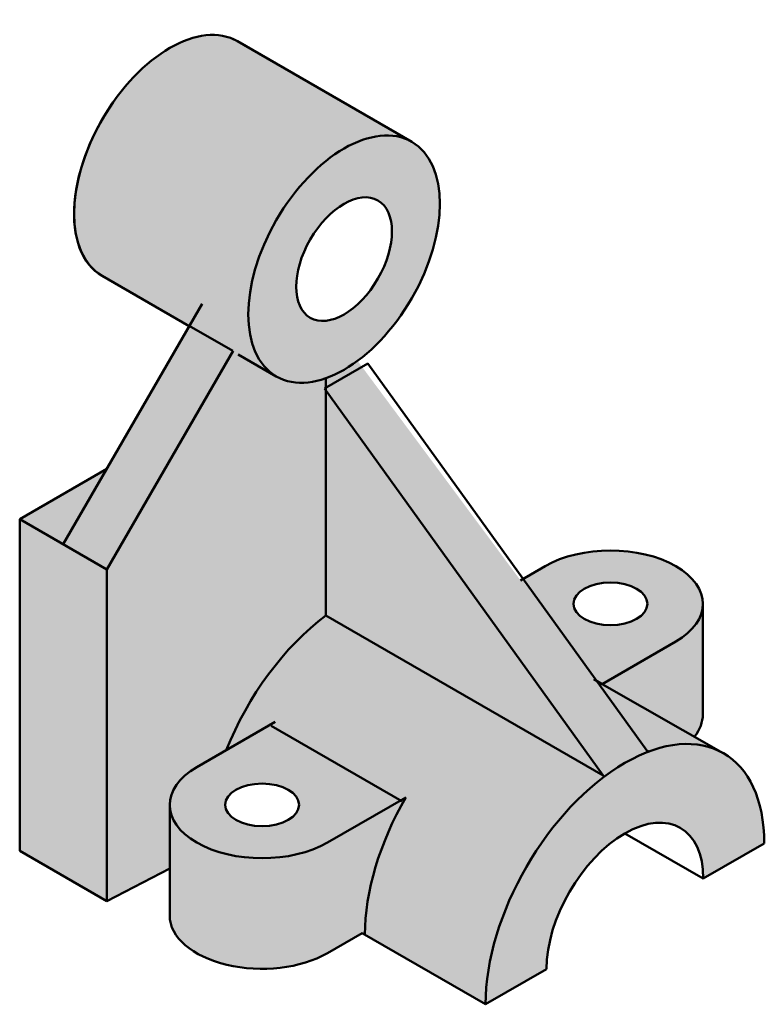
# Model space of a CAD drawing. Units: millimetres. Extents: x 293 to 441, y 10 to 206.
import ezdxf

# ---------------------------------------------------------------- set-up
doc = ezdxf.new("R2010")
doc.units = ezdxf.units.MM
doc.header["$MEASUREMENT"] = 0
doc.layers.add('M-HATC', color=7, linetype='Continuous', lineweight=18)
doc.layers.add('M-OUTL', color=7, linetype='Continuous', lineweight=50)

msp = doc.modelspace()

# ---------------------------------------------------------------- hatches: boundary and pattern name
at = {"layer": 'M-HATC'}
h = msp.add_hatch(color=256, dxfattribs=at)
h.set_gradient(color1=(99, 100, 102), name='SPHERICAL')
edge = h.paths.add_edge_path()
edge.add_ellipse((331.2474804631748, 173.1151396099691), major_axis=(-13.47219358530749, -23.33452377915608), ratio=0.5773502691896261, start_angle=180, end_angle=360, ccw=False)
edge.add_line((344.7196740484819, 196.4496633891253), (336.0594200106379, 201.4496633891251))
edge.add_line((336.0594200106379, 201.4496633891251), (334.7812085243488, 202.059255185664))
edge.add_ellipse((322.5872264253303, 178.115139609969), major_axis=(-13.47219358530749, -23.33452377915608), ratio=0.5773502691896261, start_angle=183.0116922743832, end_angle=260.9194711808092)
edge.add_ellipse((322.5872264253303, 178.115139609969), major_axis=(-13.47219358530749, -23.33452377915608), ratio=0.5773502691896261, start_angle=260.9194711808092, end_angle=270.1230012647001)
edge.add_ellipse((322.5872264253303, 178.115139609969), major_axis=(-13.47219358530749, -23.33452377915608), ratio=0.5773502691896261, start_angle=270.1230012647001, end_angle=281.4665730866499)
edge.add_ellipse((322.5872264253303, 178.115139609969), major_axis=(-13.47219358530749, -23.33452377915608), ratio=0.5773502691896261, start_angle=281.4665730866499, end_angle=358.2014821927166)
edge.add_line((308.4032823361824, 155.2374582470078), (309.1150327994311, 154.7806158555397))
edge.add_ellipse((322.5872264253303, 178.115139609969), major_axis=(-13.47219358530749, -23.33452377915608), ratio=0.5773502691896261, start_angle=358.2014821927166, end_angle=360)
edge.add_line((309.1150328400221, 154.7806158308134), (317.7752868778678, 149.7806158308127))
h = msp.add_hatch(color=256, dxfattribs=at)
h.set_gradient(color1=(99, 100, 102), name='HEMISPHERICAL')
edge = h.paths.add_edge_path()
edge.add_ellipse((349.6727660847405, 162.4772959964623), major_axis=(-13.47219358530749, -23.33452377915608), ratio=0.577350269189626, start_angle=180, end_angle=327.38609714959375, ccw=False)
edge.add_line((363.144959670048, 185.8118197756184), (344.7196740484819, 196.4496633891253))
edge.add_ellipse((331.2474804631748, 173.1151396099691), major_axis=(-13.47219358530749, -23.33452377915608), ratio=0.5773502691896261, start_angle=180, end_angle=360)
edge.add_line((317.7752868778677, 149.7806158308127), (326.4355409157117, 144.780615830813))
edge.add_line((326.4355409157117, 144.780615830813), (328.977991237339, 149.1842689635913))
edge.add_line((328.977991237339, 149.1842689635913), (330.6452880858972, 152.6202450327163))
edge = h.paths.add_edge_path()
edge.add_ellipse((357.2282425767079, 158.1151396099691), major_axis=(-13.47219358530749, -23.33452377915608), ratio=0.577350269189626, start_angle=37.55879179640515, end_angle=180)
edge.add_ellipse((357.2282425767079, 158.1151396099691), major_axis=(-13.47219358530749, -23.33452377915608), ratio=0.577350269189626, start_angle=180, end_angle=360)
edge.add_ellipse((357.2282425767079, 158.1151396099691), major_axis=(-13.47219358530749, -23.33452377915608), ratio=0.577350269189626, start_angle=3.8e-15, end_angle=21.31727217983122)
edge.add_ellipse((357.2282425767079, 158.1151396099691), major_axis=(-13.47219358530749, -23.33452377915608), ratio=0.577350269189626, start_angle=21.31727217983122, end_angle=37.55879179640515)
edge = h.paths.add_edge_path(flags=16)
edge.add_ellipse((357.2282425767079, 158.1151396099691), major_axis=(-6.736096792653745, -11.66726188957804), ratio=0.577350269189626, start_angle=0, end_angle=360)
edge = h.paths.add_edge_path()
edge.add_ellipse((357.2282425767079, 158.1151396099691), major_axis=(-13.47219358530749, -23.33452377915608), ratio=0.577350269189626, start_angle=180, end_angle=360, ccw=False)
edge.add_line((370.7004361620154, 181.4496633891251), (363.144959670048, 185.8118197756184))
edge.add_ellipse((349.6727660847405, 162.4772959964623), major_axis=(-13.47219358530749, -23.33452377915608), ratio=0.577350269189626, start_angle=180, end_angle=327.3860971495937)
edge.add_ellipse((349.6727660847405, 162.4772959964623), major_axis=(-13.47219358530749, -23.33452377915608), ratio=0.577350269189626, start_angle=327.3860971495937, end_angle=357.3493787964633)
edge.add_ellipse((349.6727660847405, 162.4772959964623), major_axis=(-13.47219358530749, -23.33452377915608), ratio=0.577350269189626, start_angle=357.3493787964633, end_angle=360)
edge.add_line((336.2005724994323, 139.1427722173067), (343.7560489914003, 134.7806158308131))
edge = h.paths.add_edge_path()
edge.add_ellipse((410.2014188270746, 89.5310620419904), major_axis=(-18.37117307087389, 0), ratio=0.5773502691896255, start_angle=150, end_angle=180)
edge.add_ellipse((410.2014188270746, 89.5310620419904), major_axis=(-18.37117307087389, 0), ratio=0.5773502691896255, start_angle=180, end_angle=330)
edge.add_line((397.2110377703077, 97.0310620419904), (392.3114166250812, 94.20226445486657))
edge.add_line((392.3114166250812, 94.20226445486657), (406.8915387662745, 74.54425491484633))
edge.add_line((406.8915387662745, 74.54425491484633), (408.5579041597167, 73.58217840637418))
edge.add_line((408.5579041597167, 73.58217840637418), (423.1917998838415, 82.03106204199057))
edge = h.paths.add_edge_path(flags=16)
edge.add_ellipse((410.2014188270746, 89.5310620419904), major_axis=(-7.348469228349532, 0), ratio=0.5773502691896266, start_angle=0, end_angle=360)
edge = h.paths.add_edge_path()
edge.add_line((343.517462735673, 66.03106204199042), (327.9290054675531, 57.03106204199063))
edge.add_ellipse((340.9193865243195, 49.53106204199039), major_axis=(-18.37117307087383, 0), ratio=0.577350269189626, start_angle=330, end_angle=360)
edge.add_ellipse((340.9193865243195, 49.53106204199039), major_axis=(-18.37117307087383, 0), ratio=0.577350269189626, start_angle=360, end_angle=510)
edge.add_line((353.9097675810864, 42.03106204199056), (369.4982248492062, 51.03106204199045))
edge.add_line((369.4982248492062, 51.03106204199045), (343.517462735673, 66.03106204199042))
edge = h.paths.add_edge_path(flags=16)
edge.add_ellipse((340.9193865243195, 49.53106204199039), major_axis=(-7.348469228349532, 0), ratio=0.5773502691896266, start_angle=0, end_angle=360)
h = msp.add_hatch(color=256, dxfattribs=at)
h.set_gradient(color1=(99, 100, 102), tint=1, name='INVCYLINDER')
edge = h.paths.add_edge_path()
edge.add_ellipse((357.2282425767079, 158.1151396099691), major_axis=(-13.47219358530749, -23.33452377915608), ratio=0.577350269189626, start_angle=0, end_angle=21.31727217983132, ccw=False)
edge.add_line((343.7560489914004, 134.780615830813), (336.2005724994323, 139.1427722173067))
edge.add_ellipse((349.6727660847405, 162.4772959964623), major_axis=(-13.47219358530749, -23.33452377915608), ratio=0.577350269189626, start_angle=357.3493787964634, end_angle=360, ccw=False)
edge.add_line((335.1668580800665, 139.8391305372528), (334.4186373269169, 138.6077444167414))
edge.add_line((334.4186373269169, 138.6077444167414), (310.0455646233283, 96.39234415755584))
edge.add_line((310.0455646233283, 96.39234415755584), (310.0455646233283, 30.39234415755584))
edge.add_line((310.0455646233283, 30.39234415755584), (322.5482134534457, 36.90721969717821))
edge.add_line((322.5482134534457, 36.90721969717821), (322.5482134534457, 49.5310620419904))
edge.add_ellipse((340.9193865243195, 49.53106204199039), major_axis=(-18.37117307087383, 0), ratio=0.577350269189626, start_angle=330, end_angle=360, ccw=False)
edge.add_line((327.9290054675533, 57.03106204199066), (333.8044668237333, 60.42326123759435))
edge.add_ellipse((357.6455487257279, 57.87420779249806), major_axis=(-19.59591794226541, -33.94112549695428), ratio=0.5773502691896261, start_angle=217.8329529862252, end_angle=293.8972038268473, ccw=False)
edge.add_line((353.6107192245012, 87.20371769116547), (353.6107192245012, 134.4267613816653))
h.paths.add_polyline_path([(310.0455646233283, 96.39234415755584), (292.7250565476396, 106.3923441575558), (292.7250565476396, 40.39234415755584), (310.0455646233283, 30.39234415755584)])
edge = h.paths.add_edge_path()
edge.add_line((334.4186373269169, 138.6077444167414), (335.1668580800665, 139.8391305372528))
edge.add_ellipse((349.6727660847405, 162.4772959964623), major_axis=(-13.47219358530749, -23.33452377915608), ratio=0.577350269189626, start_angle=327.38609714959375, end_angle=357.3493787964634, ccw=False)
edge.add_line((330.6452880858972, 152.6202450327163), (328.977991237339, 149.1842689635913))
edge.add_line((328.977991237339, 149.1842689635913), (301.385310585484, 101.3923441575558))
edge.add_line((301.385310585484, 101.3923441575558), (310.0455646233283, 96.39234415755584))
edge.add_line((310.0455646233283, 96.39234415755584), (334.4186373269169, 138.6077444167414))
h.paths.add_polyline_path([(310.0455646233284, 116.3923441575558), (292.7250565476396, 106.3923441575558), (301.385310585484, 101.3923441575558)])
h = msp.add_hatch(color=256, dxfattribs=at)
h.set_gradient(color1=(99, 100, 102), tint=1)
edge = h.paths.add_edge_path()
edge.add_ellipse((389.0941427914715, 39.71735354300563), major_axis=(-19.59591794226541, -33.94112549695428), ratio=0.5773502691896261, start_angle=270, end_angle=329.9999999999999)
edge.add_line((361.3813298703695, 23.71735354300568), (385.3583616468298, 9.874207792498083))
edge.add_ellipse((413.0711745679318, 25.87420779249803), major_axis=(-19.59591794226541, -33.94112549695428), ratio=0.5773502691896261, start_angle=217.8329529862252, end_angle=329.99999999999994, ccw=False)
edge.add_line((409.0363450667052, 55.20371769116547), (408.7410475490096, 55.37420779249803))
edge.add_line((408.7410475490096, 55.37420779249803), (353.6107192245012, 87.20371769116544))
edge.add_ellipse((357.6455487257279, 57.87420779249806), major_axis=(-19.59591794226541, -33.94112549695428), ratio=0.5773502691896261, start_angle=217.8329529862252, end_angle=293.8972038268473)
edge.add_line((333.8044668237333, 60.42326123759435), (343.517462735673, 66.03106204199041))
edge.add_line((343.517462735673, 66.03106204199041), (369.4982248492062, 51.03106204199045))
edge = h.paths.add_edge_path()
edge.add_ellipse((413.0711745679318, 25.87420779249803), major_axis=(-11.02270384252428, -19.0918830920368), ratio=0.5773502691896267, start_angle=150, end_angle=329.99999999999994, ccw=False)
edge.add_line((428.6596318360517, 34.87420779249803), (440.7839874890338, 41.87420779249802))
edge.add_ellipse((413.0711745679318, 25.87420779249803), major_axis=(-19.59591794226541, -33.94112549695428), ratio=0.5773502691896261, start_angle=149.9999999999999, end_angle=329.9999999999999)
edge.add_line((385.3583616468298, 9.874207792498026), (397.482717299812, 16.87420779249803))
edge = h.paths.add_edge_path()
edge.add_ellipse((357.2282425767079, 158.1151396099691), major_axis=(-13.47219358530749, -23.33452377915608), ratio=0.577350269189626, start_angle=21.31727217983132, end_angle=37.55879179640522, ccw=False)
edge.add_line((353.6107192245011, 134.4267613816652), (409.8052146819296, 55.76560936360246))
edge.add_ellipse((413.0711745679318, 25.87420779249803), major_axis=(-19.59591794226541, -33.94112549695428), ratio=0.5773502691896261, start_angle=202.1268965806604, end_angle=216.2354511619722, ccw=False)
edge.add_line((417.8093604415471, 60.13861490289572), (417.401301586854, 60.37420779249802))
edge.add_line((417.401301586854, 60.37420779249802), (359.9127737868367, 137.8845343172361))
h = msp.add_hatch(color=256, dxfattribs=at)
h.set_gradient(color1=(99, 100, 102), tint=1, name='INVHEMISPHERICAL')
edge = h.paths.add_edge_path()
edge.add_line((353.6107192245012, 134.4267613816652), (353.6107192245012, 87.20371769116544))
edge.add_line((353.6107192245012, 87.20371769116544), (408.7410475490096, 55.37420779249806))
edge.add_line((408.7410475490096, 55.37420779249806), (409.0363450667052, 55.20371769116547))
edge.add_ellipse((413.0711745679318, 25.87420779249803), major_axis=(-19.59591794226541, -33.94112549695428), ratio=0.5773502691896261, start_angle=216.2354511619722, end_angle=217.8329529862252, ccw=False)
edge.add_line((409.8052146819296, 55.76560936360245), (353.6107192245012, 134.4267613816652))
h = msp.add_hatch(color=256, dxfattribs=at)
h.set_gradient(color1=(99, 100, 102), tint=1, name='CYLINDER')
edge = h.paths.add_edge_path()
edge.add_ellipse((340.9193865243195, 49.53106204199039), major_axis=(-18.37117307087383, 0), ratio=0.577350269189626, start_angle=360, end_angle=510, ccw=False)
edge.add_line((322.5482134534457, 49.53106204199039), (322.5482134534457, 27.5310620419904))
edge.add_ellipse((340.9193865243195, 27.5310620419904), major_axis=(-18.37117307087383, 0), ratio=0.577350269189626, start_angle=360, end_angle=510)
edge.add_line((353.9097675810868, 20.03106204199078), (360.8379708113617, 24.03106204199043))
edge.add_line((360.8379708113617, 24.03106204199043), (361.3813298703695, 23.71735354300568))
edge.add_ellipse((389.0941427914715, 39.71735354300563), major_axis=(-19.59591794226541, -33.94112549695428), ratio=0.5773502691896261, start_angle=270, end_angle=329.99999999999994, ccw=False)
edge.add_line((369.4982248492061, 51.03106204199043), (353.9097675810865, 42.03106204199063))
edge = h.paths.add_edge_path()
edge.add_ellipse((410.2014188270746, 89.5310620419904), major_axis=(-18.37117307087389, 0), ratio=0.5773502691896255, start_angle=150, end_angle=180, ccw=False)
edge.add_line((423.1917998838413, 82.0310620419904), (408.5579041597165, 73.58217840637411))
edge.add_line((408.5579041597165, 73.58217840637411), (426.899643074779, 63.10879614566539))
edge.add_ellipse((410.2014188270746, 67.5310620419904), major_axis=(-18.37117307087389, 0), ratio=0.5773502691896255, start_angle=165.1666334603066, end_angle=180)
edge.add_line((428.5725918979484, 67.53106204198984), (428.5725918979484, 89.53106204199))
h = msp.add_hatch(color=256, dxfattribs=at)
h.set_gradient(color1=(99, 100, 102), tint=1, name='HEMISPHERICAL')
edge = h.paths.add_edge_path()
edge.add_line((408.5579041597338, 73.58217840636426), (406.8915387662745, 74.54425491484633))
edge.add_line((406.8915387662745, 74.54425491484633), (417.401301586854, 60.37420779249803))
edge.add_line((417.401301586854, 60.37420779249803), (417.8093604415472, 60.13861490289572))
edge.add_ellipse((413.0711745679318, 25.87420779249803), major_axis=(-19.59591794226541, -33.94112549695428), ratio=0.5773502691896261, start_angle=180.0910158425441, end_angle=202.1268965806604, ccw=False)
edge.add_line((432.613102131739, 59.84633335456605), (408.5579041597338, 73.58217840636426))

# ---------------------------------------------------------------- linework, layer by layer
at = {"layer": 'M-OUTL'}
for p, q in [((336.0594200106378, 201.4496633891251), (334.7812085243486, 202.0592551856641)), ((336.0594200106378, 201.4496633891251), (370.7004361620154, 181.4496633891251)), ((343.2610605988803, 197.2917942568964), (336.0594200106378, 201.4496633891251)), ((309.1150328394636, 154.7806158298444), (308.403282316191, 155.2374582598394)), ((309.1150328400229, 154.780615830813), (326.4355409157117, 144.780615830813)), ((317.2471182342343, 150.085554139392), (309.1150328394636, 154.7806158298444)), ((301.385310585484, 101.3923441575558), (328.977991237339, 149.1842689635913)), ((335.1101107537969, 139.83773795561), (326.4498567159525, 144.83773795561)), ((334.4186373269169, 138.6077444167412), (335.1668580800665, 139.8391305372529)), ((343.7560489914005, 134.780615830813), (336.2005724994331, 139.1427722173063)), ((310.0455646233283, 96.39234415755584), (334.4186373269169, 138.6077444167412)), ((353.3175801343601, 132.374), (361.9778341722045, 137.374)), ((361.9778341722045, 137.374), (417.4034600144087, 60.374)), ((353.6107192245012, 87.20371769116544), (353.6107192245012, 134.4267613816652)), ((353.3175801343601, 132.374), (408.7432059765642, 55.37400000000001)), ((292.7250565476396, 106.3923441575558), (310.0455646233283, 116.3923441575558)), ((310.0455646233283, 96.39234415755584), (292.7250565476396, 106.3923441575558)), ((292.7250565476396, 106.3923441575558), (292.7250565476396, 40.39234415755583)), ((310.0455646233283, 30.39234415755583), (310.0455646233283, 96.39234415755584)), ((397.2110377703079, 97.03106204199042), (392.3114166250811, 94.20226445486655)), ((428.5725918979484, 67.5310620419904), (428.5725918979484, 89.5310620419904)), ((408.7410475490096, 55.37420779249806), (353.6107192245012, 87.20371769116544)), ((423.1917998838412, 82.03106204199035), (408.5579041597167, 73.58217840637417)), ((408.5579041597167, 73.58217840637417), (406.8915387662744, 74.54425491484639)), ((408.5579041597165, 73.58217840637413), (432.6131021317392, 59.84633335456599)), ((327.9290054675529, 57.03106204199039), (343.517462735673, 66.03106204199042)), ((342.7192477784909, 65.25504996137774), (368.700009892024, 50.25504996137773)), ((417.401301586854, 60.37420779249803), (417.8093604415472, 60.13861490289571)), ((408.7410475490096, 55.37420779249803), (409.0363450667052, 55.20371769116542)), ((353.9097675810861, 42.03106204199039), (369.4982248492061, 51.0310620419904)), ((322.5482134534457, 27.5310620419904), (322.5482134534457, 49.53106204199039)), ((428.6617902636063, 34.87399999999999), (413.0733329954863, 43.87399999999998)), ((428.6596318360517, 34.87420779249803), (440.7839874890339, 41.87420779249805)), ((428.6596318360517, 34.87420779249803), (440.7839874890338, 41.874207792498)), ((292.7250565476396, 40.39234415755583), (310.0455646233283, 30.39234415755583)), ((310.0455646233283, 30.39234415755583), (322.5482134534457, 36.9072196971782)), ((353.9097675810861, 20.03106204199037), (360.8379708113617, 24.03106204199043)), ((385.3583616468299, 9.874207792498053), (360.8379708113617, 24.03106204199043)), ((397.482717299812, 16.87420779249803), (385.3583616468297, 9.87420779249797)), ((397.482717299812, 16.87420779249803), (385.3583616468299, 9.874207792498053))]:
    msp.add_line(p, q, dxfattribs=at)
for centre, major_axis, ratio, start_param, end_param in [((322.5872264253303, 178.115139609969), (-13.47219358530748, -23.33452377915606), 0.577350269189626, 3.141592653589793, 6.283185307179586), ((322.5872264247711, 178.1151396090004), (-13.47219358530748, -23.33452377915606), 0.577350269189626, 4.516037532074538, 6.283194418822338), ((410.2014188270746, 89.5310620419904), (-18.37117307087389, 0), 0.5773502691896255, 2.356194490192344, 5.497787143782137), ((357.6455487257279, 57.87420779249806), (-19.59591794226541, -33.94112549695428), 0.577350269189626, 4.073104533225874, 4.962830907260101), ((413.0711745679318, 25.87420779249803), (-19.59591794226541, -33.94112549695428), 0.577350269189626, 2.356194490192344, 5.497787143782137), ((410.2014188270746, 67.5310620419904), (-18.37117307087389, 0), 0.5773502691896255, 2.711521775505615, 3.141592653589793), ((340.9193865243195, 49.53106204199039), (-18.37117307087383, 0), 0.577350269189626, 5.497787143782137, 8.63937979737193), ((389.0941427914715, 39.71735354300563), (-19.59591794226541, -33.94112549695428), 0.577350269189626, 4.712388980384689, 5.497787143782137), ((413.0711745679318, 25.87420779249803), (-11.02270384252428, -19.09188309203679), 0.5773502691896267, 2.356194490192344, 5.497787143782137), ((340.9193865243195, 27.5310620419904), (-18.37117307087383, 0), 0.577350269189626, 6.283185307179586, 8.63937979737193)]:
    msp.add_ellipse(centre, major_axis=major_axis, ratio=ratio, start_param=start_param, end_param=end_param, dxfattribs=at)
for centre, major_axis, ratio in [((357.2282425767079, 158.1151396099691), (-13.47219358530748, -23.33452377915606), 0.577350269189626), ((357.2282425767079, 158.1151396099691), (-6.73609679265374, -11.66726188957803), 0.577350269189626), ((410.2014188270746, 89.5310620419904), (-7.348469228349532, 0), 0.5773502691896266), ((340.9193865243195, 49.53106204199039), (-7.348469228349532, 0), 0.5773502691896266)]:
    msp.add_ellipse(centre, major_axis=major_axis, ratio=ratio, dxfattribs=at)

doc.saveas('drawing.dxf')
